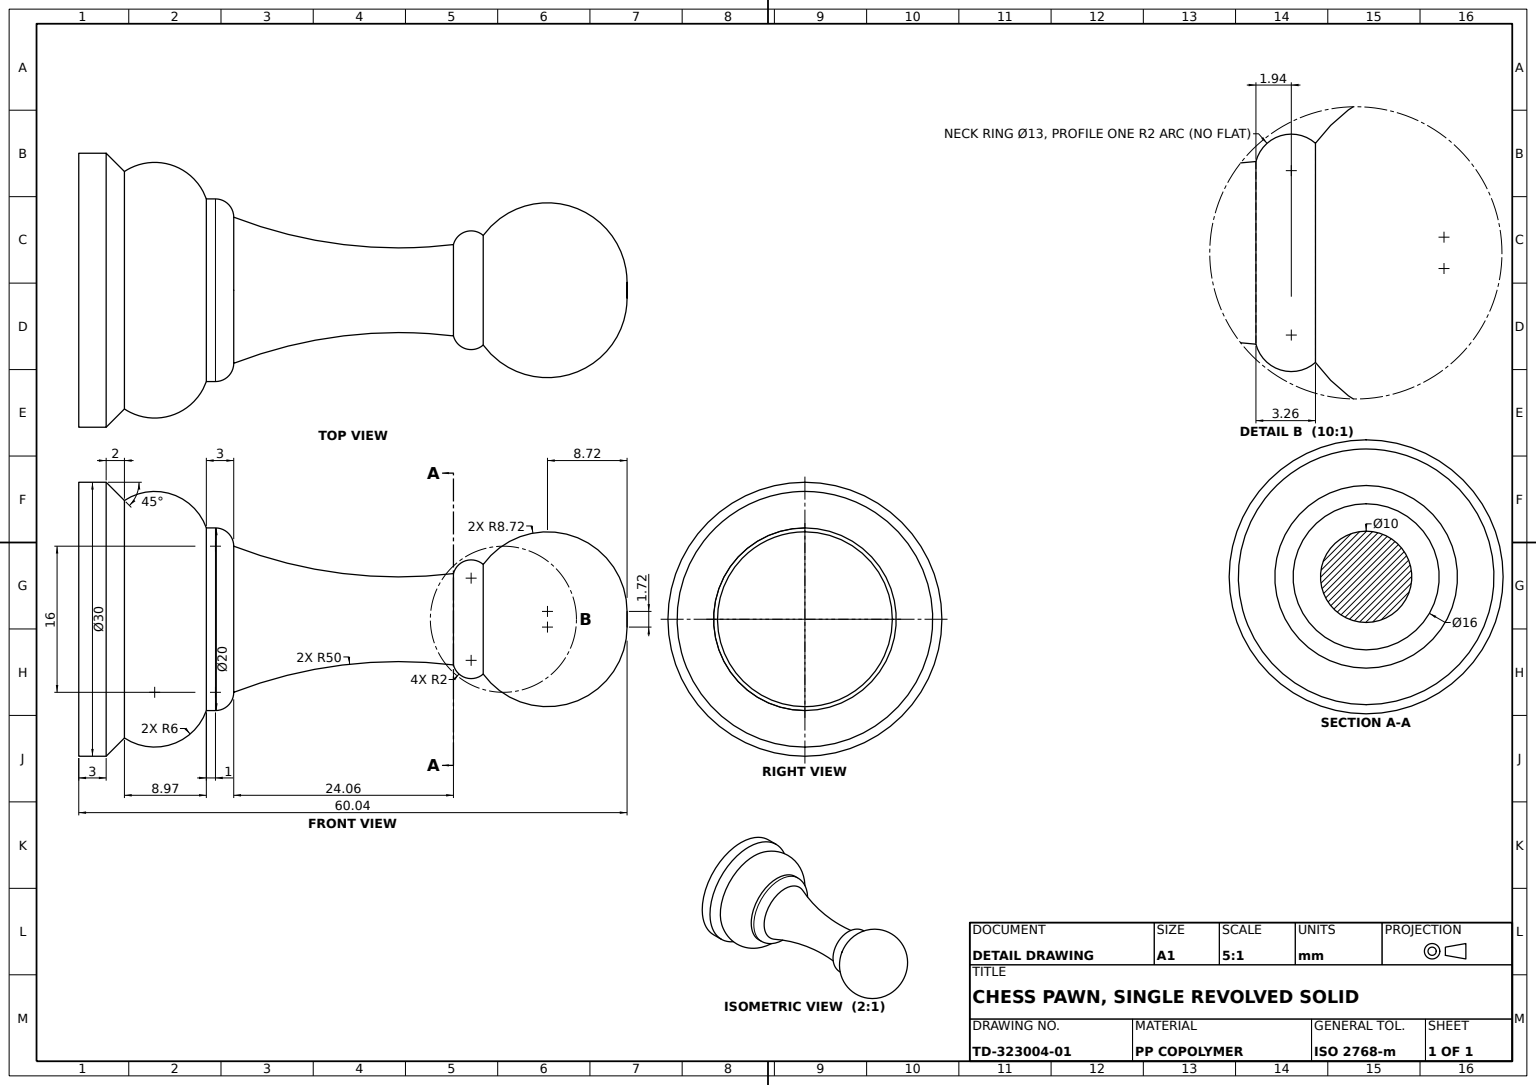
SolidWorks part; units mm, degrees
material "PP Copolymer"
ref_plane "Front Plane" through (0, 0, 0) normal (0, 0, 1) x (1, 0, 0)
ref_plane "Top Plane" through (0, 0, 0) normal (0, 1, 0) x (1, 0, 0)
ref_plane "Right Plane" through (0, 0, 0) normal (1, 0, 0) x (0, 0, -1)
sketch "Pawn Profile Sketch" plane through (0, 0, 0) normal (0, 0, 1) x (1, 0, 0)
  line L0 (0, 0) -> (0, 70.1665) construction
  line L1 (0, 0) -> (15, 0)
  line L2 (15, 0) -> (15, 3)
  line L3 (15, 3) -> (13, 5)
  line L4 (10, 13.97) -> (10, 14.97)
  line L5 (0, 0) -> (0, 60)
  arc A0 (10, 13.97) -> (13, 5) centre (7.9981, 8.3138) cw
  arc A1 (10, 14.97) -> (8, 16.97) centre (8, 14.97) ccw
  arc A2 (8, 16.97) -> (5, 41.03) centre (54.6353, 35.0019) cw
  arc A3 (5, 41.03) -> (6, 44.29) centre (4.5005, 42.9666) ccw
  arc A4 (6, 44.29) -> (0, 60) centre (0.8582, 51.327) ccw
  point P18 (9, 54.4365)
  dimension "D5" = 6
  dimension "D7" = 8.97
  dimension "D9" = 2
  dimension "D11" = 24.06
  dimension "D13" = 50
  dimension "D15" = 3.26
  dimension "D14" = 2
  dimension "D1" = 15
  dimension "D2" = 3
  dimension "D3" = 2
  dimension "D4" = 13
  dimension "D6" = 10
  dimension "D8" = 1
  dimension "D10" = 8
  dimension "D12" = 5
  dimension "D16" = 6
  dimension "D17" = 15.71
  dimension "D18" = 9
revolve "Pawn Body Revolve" add sketch "Pawn Profile Sketch" angle 360 about L0
